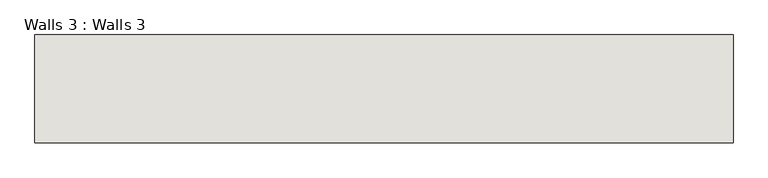
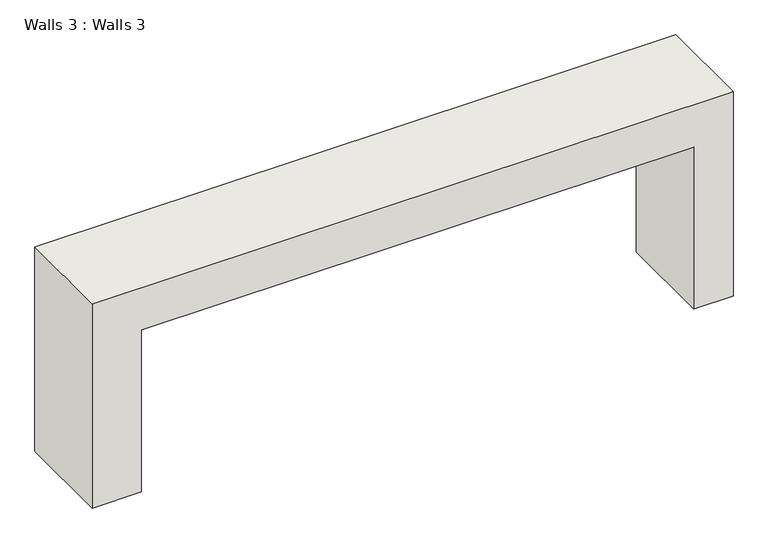
"""IFC4 building model written with IfcOpenShell, lengths in millimetres: wall geometry, Walls 3 : Walls 3."""

from ifc_helpers import new_model, si_unit, frame, origin, place, context, project, spatial, polyline, outline, extrude, source, transform, mapped, element, save


def walls_3_walls_3_d266139f(model_context):
    return source(origin(), model_context, "Body", "SweptSolid", [
        extrude(outline(polyline([(2648.0, -8498.4019361), (2648.0, 35.9980639), (0.0, 35.9980639), (0.0, 645.5980639), (3341.3717218, 645.5980639), (3341.3717218, -9260.4019361), (0.0, -9260.4019361), (0.0, -8498.4019361), (2648.0, -8498.4019361)])), frame((0.0, -7420.2562913, 0.0), z_axis=(0.0, 1.0, 0.0), x_axis=(0.0, 0.0, 1.0)), (0.0, 0.0, 1.0), 1532.724017),
    ])


if __name__ == "__main__":
    model = new_model("IFC4")
    model_context = context("Model", 3, world=origin())
    ifc_project = project(units=[si_unit("LENGTHUNIT", "METRE", prefix="MILLI")], contexts=[model_context])
    site = spatial("IfcSite", under=ifc_project)
    building = spatial("IfcBuilding", under=site)
    placement = place(None, origin())
    walls_3_walls_3_shape = walls_3_walls_3_d266139f(model_context)
    element("IfcWall", 1, ObjectType="Walls 3 : Walls 3", at=placement, inside=building, context=model_context, shape_type="MappedRepresentation", body=[
        mapped(walls_3_walls_3_shape, transform((0.0, 0.0, 0.0), x_axis=(1.0, 0.0, 0.0), y_axis=(0.0, 1.0, 0.0), z_axis=(0.0, 0.0, 1.0))),
    ])
    save(model, "model.ifc")

# Revit data of these elements
# Element 1 (IfcWall, "Walls 3 : Walls 3")
#   Materials on its faces: "Default Wall"
# Materials
#   "Default Wall": colour RGB 80 80 80, transparency 0
